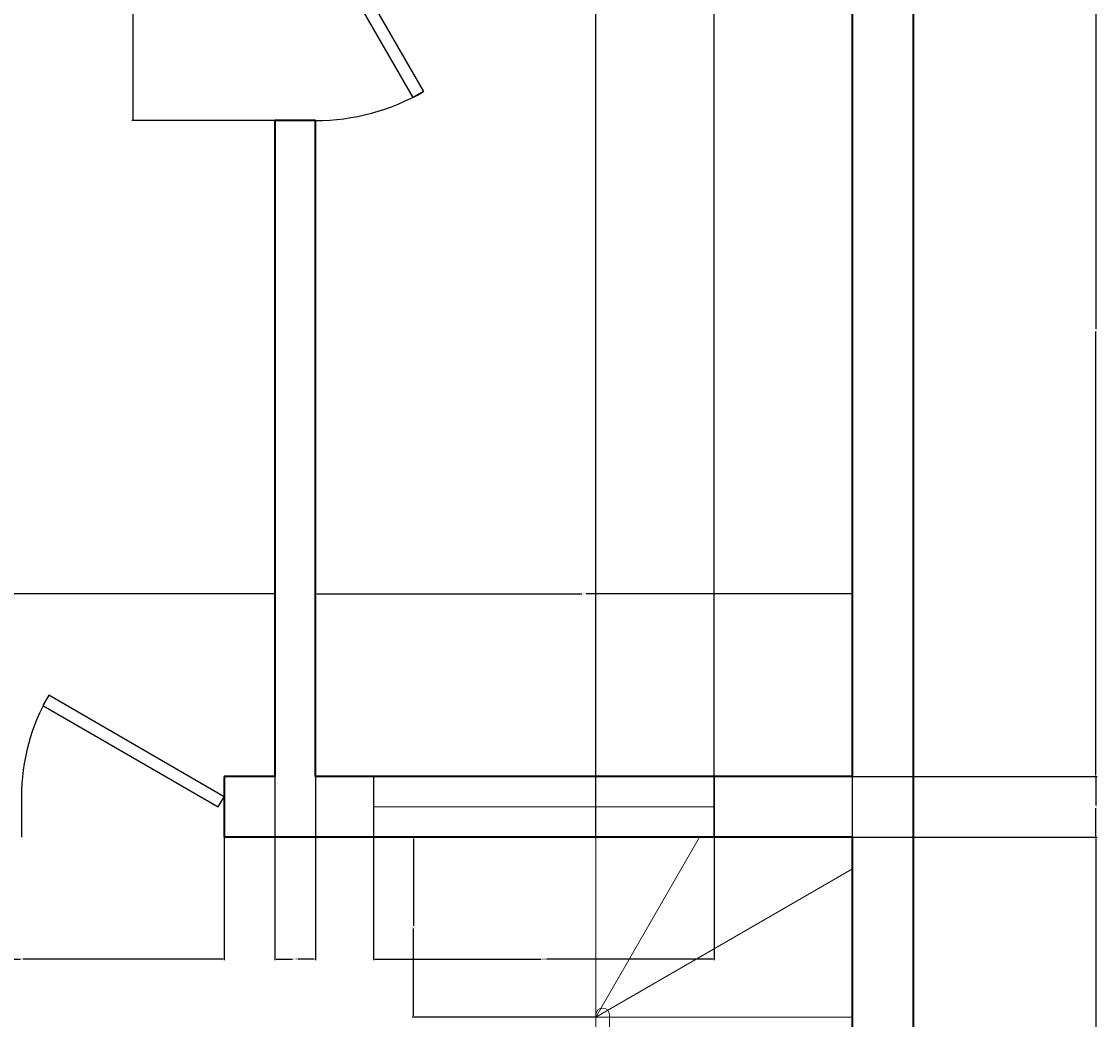
# Model space of a CAD drawing. Units: inches. Extents: x 2599 to 2953, y 557 to 1152.
# Tile 5 of 7: x 2794 to 2953, y 734 to 882. Entities that reach past the tile are written whole.
import ezdxf

# ---------------------------------------------------------------- set-up
doc = ezdxf.new("R2010")
doc.units = ezdxf.units.IN
for name, color, linetype, lineweight in [('A-ANNO-DIMS', 2, 'Continuous', 18), ('A-DOOR', 4, 'Continuous', 25), ('A-FLOR-STRS', 254, 'Continuous', 18), ('A-GLAZ', 4, 'Continuous', 18), ('A-WALL', 7, 'Continuous', 35)]:
    doc.layers.add(name, color=color, linetype=linetype, lineweight=lineweight)
doc.styles.get("Standard").update_dxf_attribs({"font": 'arial.ttf'})
doc.dimstyles.get("Standard").update_dxf_attribs({"dimtxt": 0.18, "dimasz": 0.18, "dimexe": 0.18, "dimexo": 0.0625, "dimgap": 0.09, "dimtad": 0, "dimtih": 1, "dimtoh": 1, "dimdec": 4, "dimzin": 0, "dimdsep": 46, "dimtxsty": 'Standard', "dimcen": 0.09, "dimadec": 0, "dimazin": 0, "dimtfac": 1, "dimtdec": 4, "dimtofl": 0, "dimtmove": 0, "dimatfit": 3, "dimfxl": 1, "dimtolj": 1, "dimtzin": 0, "dimarcsym": 0})

# ---------------------------------------------------------------- blocks, each defined once
blk = doc.blocks.new('*U6')
for p, q in [((0, 0), (0, -6)), ((32, 0), (32, -6))]:
    blk.add_line(p, q)
blk.add_lwpolyline([(0, 0), (27.71, 16), (28.59, 14.48), (0.87, -1.52)], close=True)
blk.add_arc((0, 0), 32, 0, 30)
blk = doc.blocks.new('*U3')
for p, q in [((-30, 0), (-30, -6)), ((0, 0), (0, -6))]:
    blk.add_line(p, q)
blk.add_lwpolyline([(0, 0), (-25.98, 15), (-26.86, 13.48), (-0.88, -1.52)], close=True)
blk.add_arc((0, 0), 30, 150, 180)
blk = doc.blocks.new('*D21')
at = {"layer": 'A-ANNO-DIMS', "color": 0, "lineweight": -2, "transparency": 16777216}
for p, q in [((2625.92, 1124.28), (2625.92, 557.16)), ((2925.92, 584.28), (2925.92, 557.16)), ((2626.1, 557.34), (2775.63, 557.34)), ((2925.74, 557.34), (2776.21, 557.34))]:
    blk.add_line(p, q, dxfattribs=at)
at = {"layer": 'A-ANNO-DIMS', "color": 0, "transparency": 16777216}
for points in [[(2626.1, 557.37), (2626.1, 557.31), (2625.92, 557.34)], [(2925.74, 557.37), (2925.74, 557.31), (2925.92, 557.34)]]:
    blk.add_solid(points, dxfattribs=at)
at = {"layer": 'Defpoints', "color": 0, "transparency": 16777216}
for p in [(2625.92, 1124.34), (2925.92, 584.34), (2925.92, 557.34)]:
    blk.add_point(p, dxfattribs=at)
at = {"layer": 'A-ANNO-DIMS', "color": 0, "transparency": 16777216, "insert": (2775.92, 557.34), "char_height": 0.18, "attachment_point": 5}
blk.add_mtext('\\A1;300', dxfattribs=at)
blk = doc.blocks.new('*D23')
at = {"layer": 'A-ANNO-DIMS', "color": 0, "lineweight": -2, "transparency": 16777216}
for p, q in [((2634.92, 770.4), (2634.92, 797.53)), ((2635.1, 797.35), (2732.79, 797.35)), ((2831.24, 797.35), (2733.56, 797.35)), ((2831.42, 770.4), (2831.42, 797.53))]:
    blk.add_line(p, q, dxfattribs=at)
at = {"layer": 'A-ANNO-DIMS', "color": 0, "transparency": 16777216}
for points in [[(2635.1, 797.38), (2635.1, 797.32), (2634.92, 797.35)], [(2831.24, 797.38), (2831.24, 797.32), (2831.42, 797.35)]]:
    blk.add_solid(points, dxfattribs=at)
at = {"layer": 'Defpoints', "color": 0, "transparency": 16777216}
for p in [(2831.42, 797.35), (2634.92, 770.34), (2831.42, 770.34)]:
    blk.add_point(p, dxfattribs=at)
at = {"layer": 'A-ANNO-DIMS', "color": 0, "transparency": 16777216, "insert": (2733.17, 797.35), "char_height": 0.18, "attachment_point": 5}
blk.add_mtext('\\A1;196.5', dxfattribs=at)
blk = doc.blocks.new('*D24')
at = {"layer": 'A-ANNO-DIMS', "color": 0, "lineweight": -2, "transparency": 16777216}
for p, q in [((2837.42, 770.4), (2837.42, 797.53)), ((2837.6, 797.35), (2876.85, 797.35)), ((2916.74, 797.35), (2877.49, 797.35)), ((2916.92, 770.4), (2916.92, 797.53))]:
    blk.add_line(p, q, dxfattribs=at)
at = {"layer": 'A-ANNO-DIMS', "color": 0, "transparency": 16777216}
for points in [[(2837.6, 797.38), (2837.6, 797.32), (2837.42, 797.35)], [(2916.74, 797.38), (2916.74, 797.32), (2916.92, 797.35)]]:
    blk.add_solid(points, dxfattribs=at)
at = {"layer": 'Defpoints', "color": 0, "transparency": 16777216}
for p in [(2916.92, 797.35), (2837.42, 770.34), (2916.92, 770.34)]:
    blk.add_point(p, dxfattribs=at)
at = {"layer": 'A-ANNO-DIMS', "color": 0, "transparency": 16777216, "insert": (2877.17, 797.35), "char_height": 0.18, "attachment_point": 5}
blk.add_mtext('\\A1;79.5', dxfattribs=at)
blk = doc.blocks.new('*D25')
at = {"layer": 'A-ANNO-DIMS', "color": 0, "lineweight": -2, "transparency": 16777216}
for p, q in [((2916.98, 902.34), (2953.1, 902.34)), ((2952.92, 902.16), (2952.92, 836.52)), ((2952.92, 770.52), (2952.92, 836.16)), ((2916.98, 770.34), (2953.1, 770.34))]:
    blk.add_line(p, q, dxfattribs=at)
at = {"layer": 'A-ANNO-DIMS', "color": 0, "transparency": 16777216}
for points in [[(2952.89, 902.16), (2952.95, 902.16), (2952.92, 902.34)], [(2952.89, 770.52), (2952.95, 770.52), (2952.92, 770.34)]]:
    blk.add_solid(points, dxfattribs=at)
at = {"layer": 'Defpoints', "color": 0, "transparency": 16777216}
for p in [(2916.92, 902.34), (2952.92, 902.34), (2916.92, 770.34)]:
    blk.add_point(p, dxfattribs=at)
at = {"layer": 'A-ANNO-DIMS', "color": 0, "transparency": 16777216, "insert": (2952.92, 836.34), "char_height": 0.18, "attachment_point": 5}
blk.add_mtext('\\A1;132', dxfattribs=at)
blk = doc.blocks.new('*D26')
at = {"layer": 'A-ANNO-DIMS', "color": 0, "lineweight": -2, "transparency": 16777216}
for p, q in [((2837.36, 899.34), (2810.24, 899.34)), ((2810.42, 899.16), (2810.42, 883.52)), ((2810.42, 867.52), (2810.42, 883.16)), ((2837.36, 867.34), (2810.24, 867.34))]:
    blk.add_line(p, q, dxfattribs=at)
at = {"layer": 'A-ANNO-DIMS', "color": 0, "transparency": 16777216}
for points in [[(2810.39, 899.16), (2810.45, 899.16), (2810.42, 899.34)], [(2810.39, 867.52), (2810.45, 867.52), (2810.42, 867.34)]]:
    blk.add_solid(points, dxfattribs=at)
at = {"layer": 'Defpoints', "color": 0, "transparency": 16777216}
for p in [(2810.42, 899.34), (2837.42, 899.34), (2837.42, 867.34)]:
    blk.add_point(p, dxfattribs=at)
at = {"layer": 'A-ANNO-DIMS', "color": 0, "transparency": 16777216, "insert": (2810.42, 883.34), "char_height": 0.18, "attachment_point": 5}
blk.add_mtext('\\A1;32', dxfattribs=at)
blk = doc.blocks.new('*D28')
at = {"layer": 'A-ANNO-DIMS', "color": 0, "lineweight": -2, "transparency": 16777216}
for p, q in [((2763.92, 770.28), (2763.92, 743.16)), ((2823.92, 770.28), (2823.92, 743.16)), ((2764.1, 743.34), (2793.7, 743.34)), ((2823.74, 743.34), (2794.14, 743.34))]:
    blk.add_line(p, q, dxfattribs=at)
at = {"layer": 'A-ANNO-DIMS', "color": 0, "transparency": 16777216}
for points in [[(2764.1, 743.37), (2764.1, 743.31), (2763.92, 743.34)], [(2823.74, 743.37), (2823.74, 743.31), (2823.92, 743.34)]]:
    blk.add_solid(points, dxfattribs=at)
at = {"layer": 'Defpoints', "color": 0, "transparency": 16777216}
for p in [(2763.92, 770.34), (2823.92, 770.34), (2763.92, 743.34)]:
    blk.add_point(p, dxfattribs=at)
at = {"layer": 'A-ANNO-DIMS', "color": 0, "transparency": 16777216, "insert": (2793.92, 743.34), "char_height": 0.18, "attachment_point": 5}
blk.add_mtext('\\A1;60', dxfattribs=at)
blk = doc.blocks.new('*D29')
at = {"layer": 'A-ANNO-DIMS', "color": 0, "lineweight": -2, "transparency": 16777216}
for p, q in [((2846.02, 770.28), (2846.02, 743.16)), ((2896.44, 770.28), (2896.44, 743.16)), ((2846.2, 743.34), (2870.84, 743.34)), ((2896.26, 743.34), (2871.62, 743.34))]:
    blk.add_line(p, q, dxfattribs=at)
at = {"layer": 'A-ANNO-DIMS', "color": 0, "transparency": 16777216}
for points in [[(2846.2, 743.37), (2846.2, 743.31), (2846.02, 743.34)], [(2896.26, 743.37), (2896.26, 743.31), (2896.44, 743.34)]]:
    blk.add_solid(points, dxfattribs=at)
at = {"layer": 'Defpoints', "color": 0, "transparency": 16777216}
for p in [(2846.02, 770.34), (2896.44, 770.34), (2846.02, 743.34)]:
    blk.add_point(p, dxfattribs=at)
at = {"layer": 'A-ANNO-DIMS', "color": 0, "transparency": 16777216, "insert": (2871.23, 743.34), "char_height": 0.18, "attachment_point": 5}
blk.add_mtext('\\A1;50.42', dxfattribs=at)
blk = doc.blocks.new('*D30')
at = {"layer": 'A-ANNO-DIMS', "color": 0, "lineweight": -2, "transparency": 16777216}
for p, q in [((2831.42, 770.28), (2831.42, 743.16)), ((2837.42, 770.28), (2837.42, 743.16)), ((2831.6, 743.34), (2834.03, 743.34)), ((2837.24, 743.34), (2834.82, 743.34))]:
    blk.add_line(p, q, dxfattribs=at)
at = {"layer": 'A-ANNO-DIMS', "color": 0, "transparency": 16777216}
for points in [[(2831.6, 743.37), (2831.6, 743.31), (2831.42, 743.34)], [(2837.24, 743.37), (2837.24, 743.31), (2837.42, 743.34)]]:
    blk.add_solid(points, dxfattribs=at)
at = {"layer": 'Defpoints', "color": 0, "transparency": 16777216}
for p in [(2831.42, 770.34), (2837.42, 770.34), (2831.42, 743.34)]:
    blk.add_point(p, dxfattribs=at)
at = {"layer": 'A-ANNO-DIMS', "color": 0, "transparency": 16777216, "insert": (2834.42, 743.34), "char_height": 0.18, "attachment_point": 5}
blk.add_mtext('\\A1;5.997', dxfattribs=at)
blk = doc.blocks.new('*D31')
at = {"layer": 'A-ANNO-DIMS', "color": 0, "lineweight": -2, "transparency": 16777216}
for p, q in [((2916.98, 770.34), (2953.1, 770.34)), ((2952.92, 770.16), (2952.92, 766.02)), ((2952.92, 761.52), (2952.92, 765.66)), ((2916.98, 761.34), (2953.1, 761.34))]:
    blk.add_line(p, q, dxfattribs=at)
at = {"layer": 'A-ANNO-DIMS', "color": 0, "transparency": 16777216}
for points in [[(2952.89, 770.16), (2952.95, 770.16), (2952.92, 770.34)], [(2952.89, 761.52), (2952.95, 761.52), (2952.92, 761.34)]]:
    blk.add_solid(points, dxfattribs=at)
at = {"layer": 'Defpoints', "color": 0, "transparency": 16777216}
for p in [(2916.92, 770.34), (2952.92, 770.34), (2916.92, 761.34)]:
    blk.add_point(p, dxfattribs=at)
at = {"layer": 'A-ANNO-DIMS', "color": 0, "transparency": 16777216, "insert": (2952.92, 765.84), "char_height": 0.18, "attachment_point": 5}
blk.add_mtext('\\A1;9', dxfattribs=at)
blk = doc.blocks.new('*D38')
at = {"layer": 'A-ANNO-DIMS', "color": 0, "lineweight": -2, "transparency": 16777216}
for p, q in [((2763.92, 761.4), (2763.92, 1151.53)), ((2764.1, 1151.35), (2821.14, 1151.35)), ((2878.74, 1151.35), (2821.7, 1151.35)), ((2878.92, 761.4), (2878.92, 1151.53))]:
    blk.add_line(p, q, dxfattribs=at)
at = {"layer": 'A-ANNO-DIMS', "color": 0, "transparency": 16777216}
for points in [[(2764.1, 1151.38), (2764.1, 1151.32), (2763.92, 1151.35)], [(2878.74, 1151.38), (2878.74, 1151.32), (2878.92, 1151.35)]]:
    blk.add_solid(points, dxfattribs=at)
at = {"layer": 'Defpoints', "color": 0, "transparency": 16777216}
for p in [(2878.92, 1151.35), (2763.92, 761.34), (2878.92, 761.34)]:
    blk.add_point(p, dxfattribs=at)
at = {"layer": 'A-ANNO-DIMS', "color": 0, "transparency": 16777216, "insert": (2821.42, 1151.35), "char_height": 0.18, "attachment_point": 5}
blk.add_mtext('\\A1;115', dxfattribs=at)
blk = doc.blocks.new('*D39')
at = {"layer": 'A-ANNO-DIMS', "color": 0, "lineweight": -2, "transparency": 16777216}
for p, q in [((2896.44, 761.4), (2896.44, 1151.53)), ((2896.62, 1151.35), (2906.21, 1151.35)), ((2916.74, 1151.35), (2907.14, 1151.35)), ((2916.92, 761.4), (2916.92, 1151.53))]:
    blk.add_line(p, q, dxfattribs=at)
at = {"layer": 'A-ANNO-DIMS', "color": 0, "transparency": 16777216}
for points in [[(2896.62, 1151.38), (2896.62, 1151.32), (2896.44, 1151.35)], [(2916.74, 1151.38), (2916.74, 1151.32), (2916.92, 1151.35)]]:
    blk.add_solid(points, dxfattribs=at)
at = {"layer": 'Defpoints', "color": 0, "transparency": 16777216}
for p in [(2916.92, 1151.35), (2896.44, 761.34), (2916.92, 761.34)]:
    blk.add_point(p, dxfattribs=at)
at = {"layer": 'A-ANNO-DIMS', "color": 0, "transparency": 16777216, "insert": (2906.68, 1151.35), "char_height": 0.18, "attachment_point": 5}
blk.add_mtext('\\A1;20.483', dxfattribs=at)
blk = doc.blocks.new('*D41')
at = {"layer": 'A-ANNO-DIMS', "color": 0, "lineweight": -2, "transparency": 16777216}
for p, q in [((2916.98, 761.34), (2953.1, 761.34)), ((2952.92, 761.16), (2952.92, 696.48)), ((2952.92, 631.44), (2952.92, 696.12)), ((2916.98, 631.26), (2953.1, 631.26))]:
    blk.add_line(p, q, dxfattribs=at)
at = {"layer": 'A-ANNO-DIMS', "color": 0, "transparency": 16777216}
for points in [[(2952.89, 761.16), (2952.95, 761.16), (2952.92, 761.34)], [(2952.89, 631.44), (2952.95, 631.44), (2952.92, 631.26)]]:
    blk.add_solid(points, dxfattribs=at)
at = {"layer": 'Defpoints', "color": 0, "transparency": 16777216}
for p in [(2916.92, 761.34), (2952.92, 761.34), (2916.92, 631.26)]:
    blk.add_point(p, dxfattribs=at)
at = {"layer": 'A-ANNO-DIMS', "color": 0, "transparency": 16777216, "insert": (2952.92, 696.3), "char_height": 0.18, "attachment_point": 5}
blk.add_mtext('\\A1;130.08', dxfattribs=at)
blk = doc.blocks.new('*D44')
at = {"layer": 'A-ANNO-DIMS', "color": 0, "lineweight": -2, "transparency": 16777216}
for p, q in [((2878.86, 761.34), (2851.74, 761.34)), ((2851.92, 761.16), (2851.92, 748.23)), ((2851.92, 734.93), (2851.92, 747.87)), ((2878.86, 734.75), (2851.74, 734.75))]:
    blk.add_line(p, q, dxfattribs=at)
at = {"layer": 'A-ANNO-DIMS', "color": 0, "transparency": 16777216}
for points in [[(2851.89, 761.16), (2851.95, 761.16), (2851.92, 761.34)], [(2851.89, 734.93), (2851.95, 734.93), (2851.92, 734.75)]]:
    blk.add_solid(points, dxfattribs=at)
at = {"layer": 'Defpoints', "color": 0, "transparency": 16777216}
for p in [(2851.92, 761.34), (2878.92, 761.34), (2878.92, 734.75)]:
    blk.add_point(p, dxfattribs=at)
at = {"layer": 'A-ANNO-DIMS', "color": 0, "transparency": 16777216, "insert": (2851.92, 748.05), "char_height": 0.18, "attachment_point": 5}
blk.add_mtext('\\A1;26.59', dxfattribs=at)

msp = doc.modelspace()

# ---------------------------------------------------------------- linework, layer by layer
at = {"layer": 'A-FLOR-STRS'}
for p, q in [((2878.9211, 631.2641), (2878.9211, 761.3417)), ((2878.9211, 734.7541), (2894.2714, 761.3417)), ((2878.9211, 734.7541), (2916.9211, 756.6935)), ((2878.9211, 734.7541), (2916.9211, 734.7541)), ((2880.9211, 631.2641), (2880.9211, 735.0939))]:
    msp.add_line(p, q, dxfattribs=at)
msp.add_arc((2879.9211, 735.0939), 1, 360, 180, dxfattribs=at)
at = {"layer": 'A-GLAZ'}
for p, q in [((2846.0203, 770.3417), (2846.0203, 761.3417)), ((2896.4376, 770.3417), (2896.4376, 761.3417)), ((2896.4376, 765.8417), (2846.0203, 765.8417))]:
    msp.add_line(p, q, dxfattribs=at)
at = {"layer": 'A-WALL'}
for p, q in [((2925.9211, 584.3417), (2925.9211, 1124.3417)), ((2916.9211, 770.3417), (2916.9211, 902.3417)), ((2837.4211, 867.3417), (2831.4243, 867.3417)), ((2831.4243, 867.3417), (2831.4243, 770.3417)), ((2837.4211, 770.3417), (2837.4211, 867.3417)), ((2831.4243, 770.3417), (2823.9243, 770.3417)), ((2823.9243, 770.3417), (2823.9243, 761.3417)), ((2916.9211, 770.3417), (2837.4211, 770.3417)), ((2916.9211, 761.3417), (2823.9243, 761.3417)), ((2916.9211, 610.5917), (2916.9211, 761.3417))]:
    msp.add_line(p, q, dxfattribs=at)

# ---------------------------------------------------------------- block references
at = {"layer": 'A-DOOR', "rotation": 270}
msp.add_blockref('*U6', (2837.4243, 899.3417), dxfattribs=at)
at = {"layer": 'A-DOOR'}
msp.add_blockref('*U3', (2823.9243, 767.3417), dxfattribs=at)

# ---------------------------------------------------------------- dimensions: what is measured, and where the dimension line sits
at = {"layer": 'A-ANNO-DIMS'}
for base, p1, p2, override, picture, middle in [((2878.9211, 1151.3452), (2763.9211, 761.3417), (2878.9211, 761.3417), {"dimdec": 0, "dimlfac": 1, "dimrnd": 0, "dimzin": 0, "dimdsep": 46, "dimlunit": 2}, '*D38', (2821.4211, 1151.3452)), ((2916.92111, 1151.34517), (2896.43762, 761.34167), (2916.92111, 761.34167), {"dimdec": 3, "dimlfac": 1, "dimrnd": 0, "dimzin": 0, "dimdsep": 46, "dimlunit": 2}, '*D39', (2906.67936, 1151.34517)), ((2925.9211, 557.3382), (2625.9211, 1124.3417), (2925.9211, 584.3417), {"dimdec": 0, "dimlfac": 1, "dimrnd": 0, "dimzin": 0, "dimdsep": 46, "dimlunit": 2}, '*D21', (2775.9211, 557.3382)), ((2831.4243, 797.3452), (2634.9211, 770.3417), (2831.4243, 770.3417), {"dimdec": 1, "dimlfac": 1, "dimrnd": 0, "dimzin": 0, "dimdsep": 46, "dimlunit": 2}, '*D23', (2733.1727, 797.3452)), ((2916.9211, 797.3452), (2837.4211, 770.3417), (2916.9211, 770.3417), {"dimdec": 1, "dimlfac": 1, "dimrnd": 0, "dimzin": 0, "dimdsep": 46, "dimlunit": 2}, '*D24', (2877.1711, 797.3452))]:
    dim = msp.add_linear_dim(base=base, p1=p1, p2=p2, dimstyle='Standard', override=override, dxfattribs=at)
    dim.commit()
    dim.dimension.update_dxf_attribs({"geometry": picture, "text_midpoint": middle})
for base, p1, p2, angle, override, picture, middle in [((2952.9246, 902.3417), (2916.9211, 770.3417), (2916.9211, 902.3417), 90, {"dimdec": 0, "dimlfac": 1, "dimrnd": 0, "dimzin": 0, "dimdsep": 46, "dimlunit": 2}, '*D25', (2952.9246, 836.3417)), ((2810.4176, 899.3417), (2837.4211, 867.3417), (2837.4211, 899.3417), 90, {"dimdec": 0, "dimlfac": 1, "dimrnd": 0, "dimzin": 0, "dimdsep": 46, "dimlunit": 2}, '*D26', (2810.4176, 883.3417)), ((2763.9211, 743.3382), (2823.9243, 770.3417), (2763.9211, 770.3417), 180, {"dimdec": 0, "dimlfac": 1, "dimrnd": 0, "dimzin": 0, "dimdsep": 46, "dimlunit": 2}, '*D28', (2793.9227, 743.3382)), ((2831.4243, 743.3382), (2837.4211, 770.3417), (2831.4243, 770.3417), 180, {"dimdec": 3, "dimlfac": 1, "dimrnd": 0, "dimzin": 0, "dimdsep": 46, "dimlunit": 2}, '*D30', (2834.4227, 743.3382)), ((2846.0203, 743.3382), (2896.4376, 770.3417), (2846.0203, 770.3417), 180, {"dimdec": 2, "dimlfac": 1, "dimrnd": 0, "dimzin": 0, "dimdsep": 46, "dimlunit": 2}, '*D29', (2871.229, 743.3382)), ((2952.9246, 770.3417), (2916.9211, 761.3417), (2916.9211, 770.3417), 90, {"dimdec": 0, "dimlfac": 1, "dimrnd": 0, "dimzin": 0, "dimdsep": 46, "dimlunit": 2}, '*D31', (2952.9246, 765.8417)), ((2851.9176, 761.3417), (2878.9211, 734.7541), (2878.9211, 761.3417), 90, {"dimdec": 2, "dimlfac": 1, "dimrnd": 0, "dimzin": 0, "dimdsep": 46, "dimlunit": 2}, '*D44', (2851.9176, 748.0479)), ((2952.9246, 761.3417), (2916.9211, 631.2641), (2916.9211, 761.3417), 90, {"dimdec": 2, "dimlfac": 1, "dimrnd": 0, "dimzin": 0, "dimdsep": 46, "dimlunit": 2}, '*D41', (2952.9246, 696.3029))]:
    dim = msp.add_linear_dim(base=base, p1=p1, p2=p2, angle=angle, dimstyle='Standard', override=override, dxfattribs=at)
    dim.commit()
    dim.dimension.update_dxf_attribs({"geometry": picture, "text_midpoint": middle})

doc.saveas('drawing.dxf')
